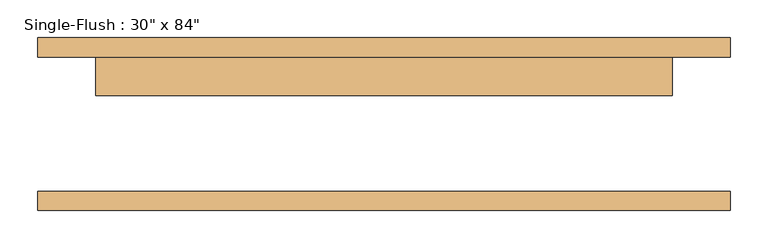
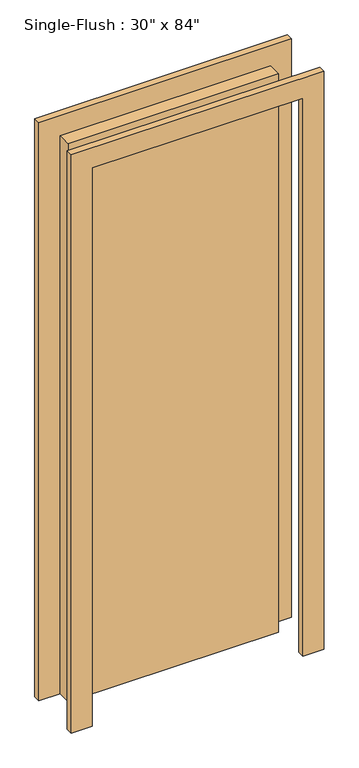
"""IFC4 building model written with IfcOpenShell, lengths in millimetres: door geometry."""

from ifc_helpers import new_model, si_unit, frame, origin, origin_with_axes, place, context, project, spatial, polyline, outline, extrude, source, transform, mapped, element, save


def door_0af0cdd0(model_context):
    return source(origin(), model_context, "Body", "SweptSolid", [
        extrude(outline(polyline([(2209.8, -457.2), (0.0, -457.2), (0.0, -381.0), (2133.6, -381.0), (2133.6, 381.0), (0.0, 381.0), (0.0, 457.2), (2209.8, 457.2), (2209.8, -457.2)])), frame((0.0, 88.9, 0.0), z_axis=(0.0, 1.0, 0.0), x_axis=(0.0, 0.0, 1.0)), (0.0, 0.0, 1.0), 25.4),
        extrude(outline(polyline([(2209.8, 457.2), (2209.8, -457.2), (0.0, -457.2), (0.0, -381.0), (2133.6, -381.0), (2133.6, 381.0), (0.0, 381.0), (0.0, 457.2), (2209.8, 457.2)])), frame((0.0, -114.3, 0.0), z_axis=(0.0, 1.0, 0.0), x_axis=(0.0, 0.0, 1.0)), (0.0, 0.0, 1.0), 25.4),
        extrude(outline(polyline([(381.0, 38.1), (-381.0, 38.1), (-381.0, 88.9), (381.0, 88.9), (381.0, 38.1)])), origin_with_axes(), (0.0, 0.0, 1.0), 2133.6),
    ])


if __name__ == "__main__":
    model = new_model("IFC4")
    model_context = context("Model", 3, world=origin())
    ifc_project = project(units=[si_unit("LENGTHUNIT", "METRE", prefix="MILLI")], contexts=[model_context])
    site = spatial("IfcSite", under=ifc_project)
    building = spatial("IfcBuilding", under=site)
    placement = place(None, origin())
    door_shape = door_0af0cdd0(model_context)
    element("IfcDoor", 1, ObjectType="Single-Flush : 30\" x 84\"", at=placement, inside=building, context=model_context, shape_type="MappedRepresentation", body=[
        mapped(door_shape, transform((0.0, 0.0, 0.0), x_axis=(1.0, 0.0, 0.0), y_axis=(0.0, 1.0, 0.0), z_axis=(0.0, 0.0, 1.0))),
    ])
    save(model, "model.ifc")

# Revit data of these elements
# Type "Single-Flush : 30\" x 84\""
#   Type Mark = "4"
#   Construction Type Id = "MDOOR"
#   Assembly Code = "C1020"
#   Analytic Construction = "Metal"
#   Thickness = 0' - 2"
#   Heat Transfer Coefficient (U) = 0.651978 BTU/(h·ft²·°F)
#   Height = 7' - 0"
#   Trim Projection Ext = 0' - 1"
#   Trim Projection Int = 0' - 1"
#   Trim Width = 0' - 3"
#   Width = 2' - 6"
#   Define Thermal Properties by = 1
#   Door Material = Door - Panel
#   Frame Material = Door - Frame
#   Visual Light Transmittance = 0
#   Solar Heat Gain Coefficient = 0
#   Function = (empty or 0)
#   Wall Closure = (empty or 0)
# Element 1 (IfcDoor, "Single-Flush : 30\" x 84\"")
#   Materials on its faces: "Door - Frame", "Door - Panel"
# Materials
#   "Door - Panel": class "Wood", colour RGB 210 159 95, transparency 0
#   "Door - Frame": colour RGB 118 70 51, transparency 0
